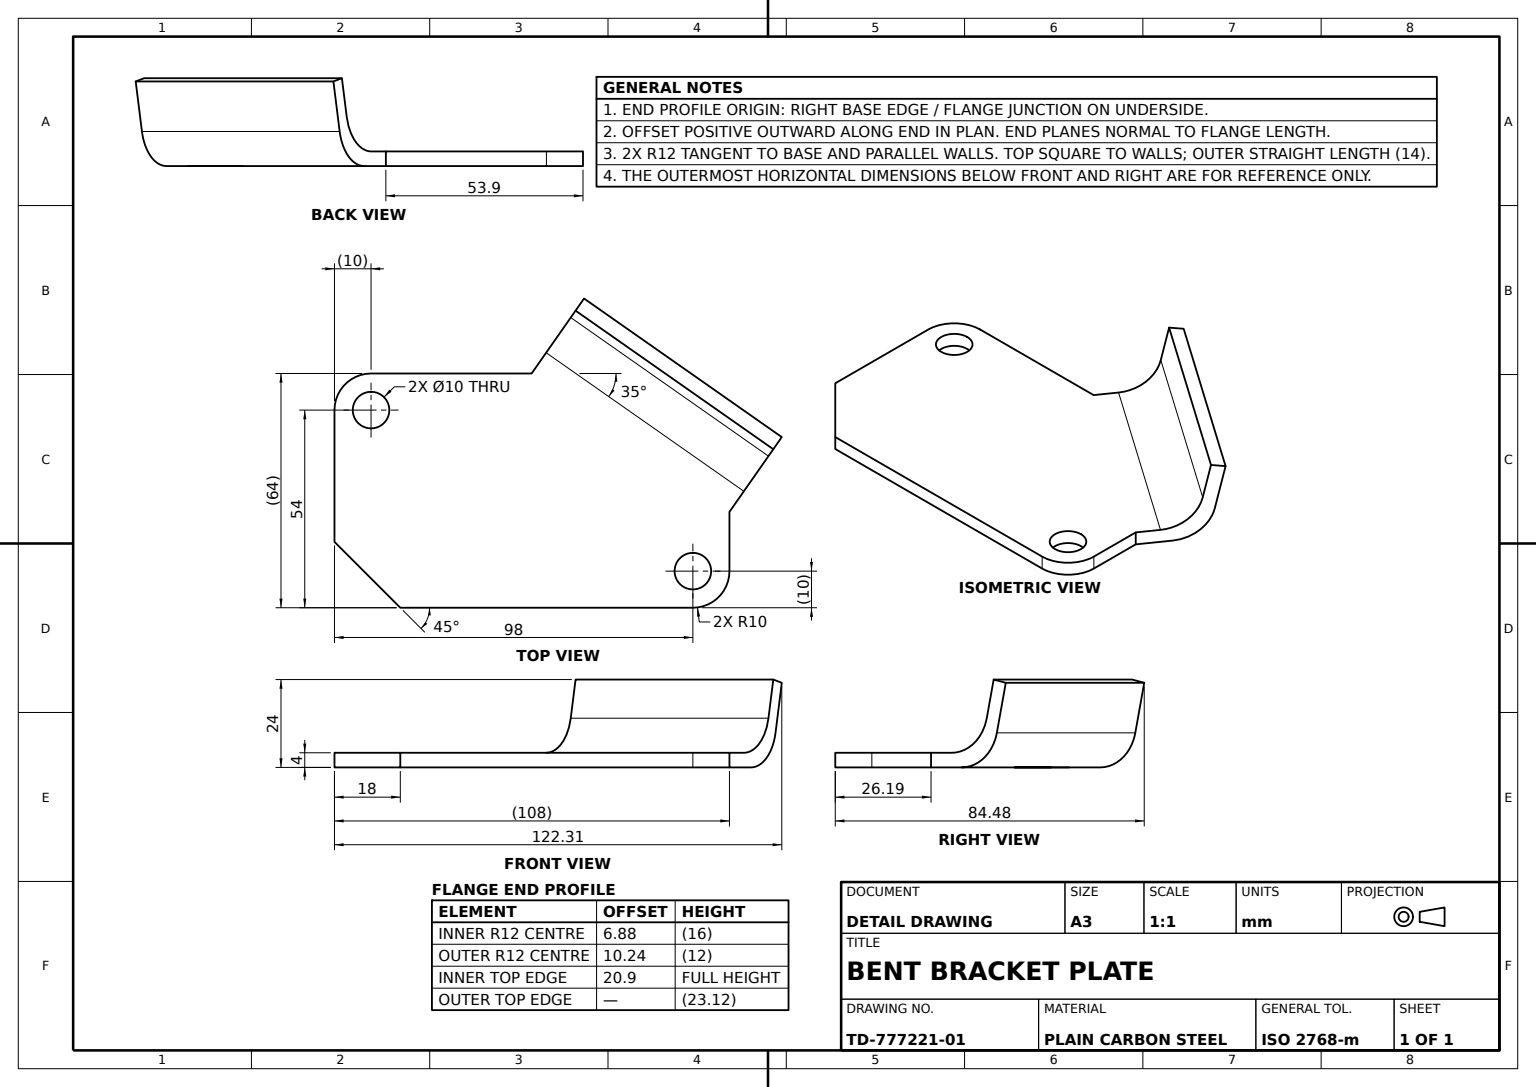
SolidWorks part; units mm, degrees
material "Plain Carbon Steel"
ref_plane "Front Plane" through (0, 0, 0) normal (0, 0, 1) x (1, 0, 0)
ref_plane "Top Plane" through (0, 0, 0) normal (0, 1, 0) x (1, 0, 0)
ref_plane "Right Plane" through (0, 0, 0) normal (1, 0, 0) x (0, 0, -1)
sketch "Base Plate Sketch" plane through (0, 0, 0) normal (0, 1, 0) x (1, 0, 0)
  line L0 (0, 32) -> (54, -5.8112)
  line L1 (-54, -32) -> (54, -32)
  line L2 (-54, -32) -> (-54, 32)
  line L3 (-54, 32) -> (0, 32)
  line L4 (54, -32) -> (54, -5.8112)
  line L5 (0, 32) -> (17.7655, 57.3717)
  line L6 (17.7655, 57.3717) -> (71.7655, 19.5605)
  line L7 (71.7655, 19.5605) -> (54, -5.8112)
  point P0 (0, 0)
  dimension "D1" = 64
  dimension "D2" = 54
  dimension "D3" = 35
  dimension "D4" = 54
  dimension "D5" = 71.7655
  dimension "D6" = 108
  dimension "D7" = 32
extrude "Base Plate" add sketch "Base Plate Sketch" along normal blind 4 contours L1 L4 L0 L3 L2
sketch "Flange Riser Sketch" plane through (15.0351, 0, -21.4723) normal (0.5736, 0, -0.8192) x (-0.8192, 0, -0.5736)
  line L1 (-47.5674, 0) -> (18.3544, 0)
  line L2 (-47.5674, 0) -> (-47.5674, 4)
  line L3 (-47.5674, 4) -> (18.3544, 4)
  line L4 (18.3544, 0) -> (18.3544, 4)
extrude "Flange Riser" add sketch "Flange Riser Sketch" along normal blind 10
sketch "Curved Flange Profile Sketch" plane through (38.9649, 0, 27.2835) normal (0.8192, 0, 0.5736) x (0.5736, 0, -0.8192)
  line L0 (23.7204, 4) -> (33.0881, 4)
  line L1 (26.2129, 4) -> (26.2129, 0) construction
  line L2 (44.8124, 13.4422) -> (47.1164, 24.003)
  line L3 (47.1164, 24.003) -> (51.162, 23.1204)
  line L4 (51.162, 23.1204) -> (48.1779, 9.4422)
  line L5 (36.4537, 0) -> (24.2458, 0)
  line L6 (36.2129, 0) -> (26.2129, 0) construction
  line L7 (24.2458, 0) -> (23.7204, 4)
  arc A0 (36.4537, 0) -> (48.1779, 9.4422) centre (36.4537, 12) ccw
  arc A1 (33.0881, 4) -> (44.8124, 13.4422) centre (33.0881, 16) ccw
  point P15 (42.7524, 4)
  dimension "D1" = 12
  dimension "D2" = 14
  dimension "D3" = 6.8753
  dimension "D4" = 10.2408
  dimension "D5" = 16.5395
  dimension "D6" = 4
  dimension "D7" = 20.9035
  dimension "D10" = 1.9671
  dimension "D11" = 2.4925
extrude "Curved Flange" add sketch "Curved Flange Profile Sketch" against normal blind 66
fillet "Plate Corner Fillets R10" radius 10 2 edges at (-54, 2, -32) (54, 2, 32)
chamfer "Plate Corner Chamfer 18" distance 18 1 edges at (-54, 2, 32)
sketch "Mounting Holes Sketch" plane through (0, 4, 0) normal (0, 1, 0) x (1, 0, 0)
  circle A0 centre (-44, 22) radius 5
  circle A1 centre (44, -22) radius 5
  dimension "D1" = 10
  dimension "D2" = 10
extrude "Mounting Holes 2x" cut sketch "Mounting Holes Sketch" against normal blind 66
